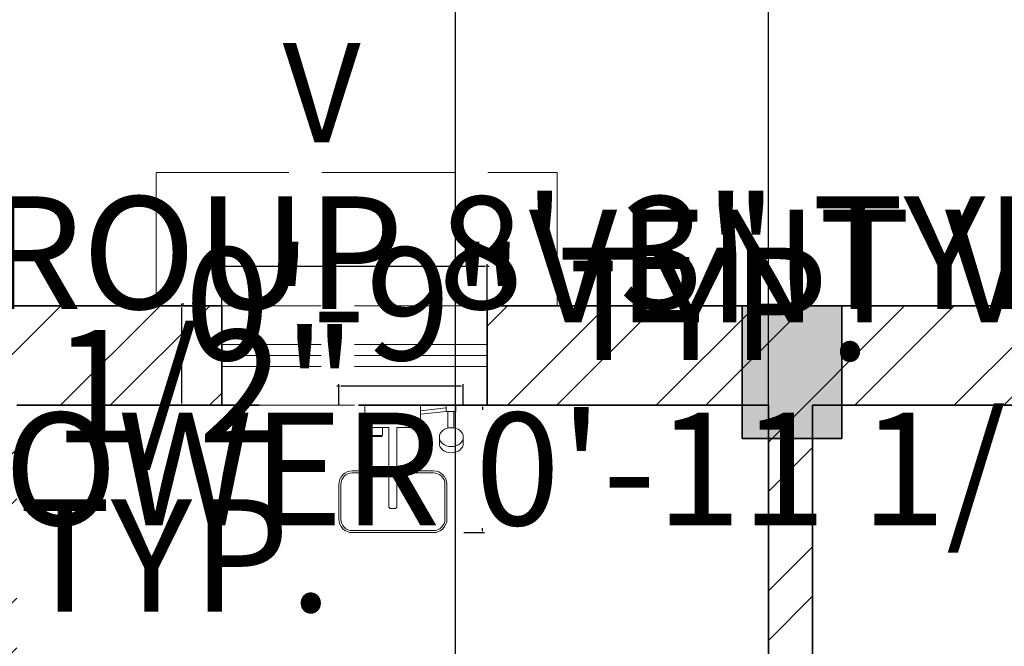
# Model space of a CAD drawing. Units: inches. Extents: x 2379 to 3013, y 1431 to 2110.
# Tile 7 of 10: x 2696 to 2785, y 1991 to 2047. Entities that reach past the tile are written whole.
import ezdxf

# ---------------------------------------------------------------- set-up
doc = ezdxf.new("R2010")
doc.units = ezdxf.units.IN
doc.linetypes.add('ACAD_ISO02W100', pattern=[15, 12, -3])
for name, color, linetype, lineweight in [('A-ANNO-DIMS', 2, 'Continuous', 18), ('A-ANNO-TEXT', 7, 'Continuous', 18), ('A-COLS', 7, 'Continuous', 35), ('A-COLS-PATT', 252, 'Continuous', 13), ('A-FLOR-FIXT', 9, 'Continuous', 18), ('A-GLAZ-VENT', 6, 'ACAD_ISO02W100', 13), ('A-ROOF-OVHD', 11, 'ACAD_ISO02W100', 13), ('A-WALL-PATT', 8, 'Continuous', 13), ('WALL', 7, 'Continuous', 35)]:
    doc.layers.add(name, color=color, linetype=linetype, lineweight=lineweight)
doc.styles.get("Standard").update_dxf_attribs({"font": 'arial.ttf'})
doc.dimstyles.get("Standard").update_dxf_attribs({"dimtxt": 10.18, "dimasz": 0.18, "dimexe": 0.18, "dimexo": 0.0625, "dimgap": 0.09, "dimtad": 0, "dimtih": 1, "dimtoh": 1, "dimdec": 0, "dimzin": 0, "dimdsep": 46, "dimlunit": 3, "dimtxsty": 'Standard', "dimcen": 0.09, "dimadec": 0, "dimazin": 0, "dimtfac": 1, "dimtdec": 0, "dimtofl": 0, "dimtmove": 0, "dimatfit": 3, "dimfxl": 1, "dimtolj": 1, "dimtzin": 0, "dimarcsym": 0})

# ---------------------------------------------------------------- blocks, each defined once
blk = doc.blocks.new('column')
for p, q in [((2588.21307907444, 2021.786762638958), (2597.21307907444, 2021.786762638958)), ((2588.21307907444, 2009.786762638958), (2588.21307907444, 2021.786762638958)), ((2597.21307907444, 2021.786762638958), (2597.21307907444, 2009.786762638958)), ((2597.21307907444, 2009.786762638958), (2588.21307907444, 2009.786762638958))]:
    blk.add_line(p, q)
blk = doc.blocks.new('A$C7A0926BE')
for p, q in [((-6.551239185704615, 4.547e-13), (-5.566804685018722, 4.547e-13)), ((-6.551239185704615, -0.6519594773226345), (-6.551239185704615, 4.547e-13)), ((-5.566804685018722, 4.547e-13), (-5.566804685018722, -0.6519594773226345)), ((-2.885464417704497, 4.547e-13), (-2.885464417704497, -2.294617439688408)), ((2.885464417697221, 4.547e-13), (-2.885464417704497, 4.547e-13)), ((2.885464417697221, -2.294617439688408), (2.885464417697221, 4.547e-13)), ((-5.566804685018722, -0.6519594773226345), (-6.551239185704615, -0.6519594773226345)), ((-6.337339280165905, -0.6519594773226345), (-5.736871956549292, -0.6519594773226345)), ((-6.337339280165905, -2.331605676014532), (-6.337339280165905, -0.6519594773226345)), ((-5.736871956549292, -0.6519594773226345), (-5.736871956549292, -2.331605676014532)), ((-5.566804685018722, -0.2752176342105486), (-2.885464417704497, -0.5594689734662098)), ((-5.566804685018722, -0.6519594773226345), (-2.885464417704497, -0.9362108165782956)), ((-5.736871956549292, -2.331605676014532), (-6.337339280165905, -2.331605676014532)), ((-2.885464417704497, -2.294617439688408), (-0.4493639847714804, -2.294617439688408)), ((0.3906360152323032, -2.294617439688408), (2.885464417697221, -2.294617439688408)), ((1.037687122458008, -2.294617439688408), (1.037687122458008, -3.123877501528568)), ((2.370543453427671, -2.294617439688408), (1.037687122458008, -2.294617439688408)), ((2.370543453427671, -3.123877501528568), (2.370543453427671, -2.294617439688408)), ((-7.324834426704909, -3.292217109228203), (-7.324834426704909, -3.941342171486666)), ((-4.843765035140676, -3.941342171486666), (-4.849446849475498, -3.292217109228203)), ((1.037687122458008, -3.123877501528568), (2.370543453427671, -3.123877501528568)), ((1.127016126156376, -3.123877501528568), (1.127016126156376, -3.234129205485259)), ((2.303627794695784, -3.123877501528568), (1.127016126156376, -3.123877501528568)), ((1.127016126156376, -3.234129205485259), (2.303627794695784, -3.234129205485259)), ((2.303627794695784, -3.234129205485259), (2.303627794695784, -3.123877501528568))]:
    blk.add_line(p, q)
at = {"ltscale": 100}
for p, q in [((-0.4493639847642045, -10.48461743968892), (-0.4493639847714804, -2.294617439688408)), ((0.3906360152323032, -10.48461743968892), (0.3906360152323032, -2.294617439688408)), ((0.1806360152259003, -10.6946174396885), (-0.2393639847723534, -10.6946174396885))]:
    blk.add_line(p, q, dxfattribs=at)
for points in [[(-0.4493639847642045, -6.794023881873727), (-4.22936398476304, -6.794023881873727, 0.4142135623730951), (-5.629363984764494, -8.194023881873362), (-5.629363984764494, -11.79521099750036, 0.4142135623730951), (-4.22936398476304, -13.19521099750091), (4.170636015231138, -13.19521099750091, 0.4142135623730951), (5.570636015232594, -11.79521099750036), (5.570636015232594, -8.194023881873362, 0.4142135623730951), (4.170636015231138, -6.794023881873727), (0.3906360152323032, -6.794023881873727)], [(-0.4493639847642045, -7.004023881873306), (-4.22936398476304, -7.004023881873306, 0.4142135623733461), (-5.419363984772644, -8.194023881873362), (-5.419363984772644, -11.79521099750036, 0.4142135623733461), (-4.22936398476304, -12.98521099750132), (4.170636015231138, -12.98521099750132, 0.4142135623733461), (5.360636015233466, -11.79521099750036), (5.360636015233466, -8.194023881873362, 0.4142135623733461), (4.170636015231138, -7.004023881873306), (0.3906360152323032, -7.004023881873306)]]:
    blk.add_lwpolyline(points, format="xyb", dxfattribs=at)
for centre, start, end in [((-0.2393639847723534, -10.48461743968892), 180, 270), ((0.1806360152259003, -10.48461743968892), 270, 0)]:
    blk.add_arc(centre, 0.2099999999999999, start, end, dxfattribs=at)
at = {"extrusion": (0, 0, -1)}
blk.add_ellipse((-6.084299730922793, -3.292217109228203), major_axis=(-1.240534695781024, -2.0763e-12), ratio=0.7908490116437874, dxfattribs=at)
blk.add_ellipse((-6.084299730922793, -3.941342171486666), major_axis=(-1.240534695781024, -1.4783e-12), ratio=0.7908490116437878, start_param=3.141592653591299, end_param=6.283185307181092, dxfattribs=at)
blk = doc.blocks.new('*D14')
at = {"layer": 'A-ANNO-DIMS', "color": 0, "lineweight": -2, "transparency": 16777216}
for p, q in [((2469.628133617025, 2021.670980178146), (2469.628133617025, 2076.343811217002)), ((2937.628133542687, 2021.670980178146), (2937.628133542687, 2076.343811217002)), ((2469.808133617025, 2076.163811217002), (2694.903188150115, 2076.163811217002)), ((2937.448133542687, 2076.163811217002), (2712.353079009597, 2076.163811217002))]:
    blk.add_line(p, q, dxfattribs=at)
at = {"layer": 'A-ANNO-DIMS', "color": 0, "transparency": 16777216}
for points in [[(2469.808133617025, 2076.193811217002), (2469.808133617025, 2076.133811217002), (2469.628133617025, 2076.163811217002)], [(2937.448133542687, 2076.193811217002), (2937.448133542687, 2076.133811217002), (2937.628133542687, 2076.163811217002)]]:
    blk.add_solid(points, dxfattribs=at)
at = {"layer": 'Defpoints', "color": 0, "transparency": 16777216}
for p in [(2937.628133542687, 2076.163811217002), (2469.628133617025, 2021.608480178145), (2937.628133542687, 2021.608480178146)]:
    blk.add_point(p, dxfattribs=at)
at = {"layer": 'A-ANNO-DIMS', "color": 0, "transparency": 16777216, "insert": (2703.628133579856, 2076.163811217002), "char_height": 10.18, "attachment_point": 5}
blk.add_mtext("\\A1;39'", dxfattribs=at)
blk = doc.blocks.new('VENT-24IN')
for p, q in [((23.99961244475026, 5.50048129934089), (-0.0003875552497448, 5.50048129934089)), ((23.99961244475026, 4.50048129934089), (-0.0003875552497448, 4.50048129934089)), ((23.99961244475026, 3.50048129934089), (-0.0003875552497448, 3.50048129934089))]:
    blk.add_line(p, q)
blk.add_lwpolyline([(-0.0003875552497448, 9.00048129910806), (-0.0003875552497448, 0.0004812991080598), (23.99961244475026, 0.0004812993408905), (23.99961244475026, 9.00048129934089)], close=True)
blk = doc.blocks.new('*D26')
at = {"layer": 'A-ANNO-DIMS', "color": 0, "lineweight": -2, "transparency": 16777216}
for p, q in [((2688.622898699378, 1958.67097978589), (2688.622898699378, 1963.759108581785)), ((2688.802898699378, 1963.579108581785), (2721.580424005343, 1963.579108581785)), ((2721.760424005343, 1958.67097978589), (2721.760424005343, 1963.759108581785)), ((2721.760424005343, 1963.579108581785), (2721.940424005343, 1963.579108581785))]:
    blk.add_line(p, q, dxfattribs=at)
at = {"layer": 'A-ANNO-DIMS', "color": 0, "transparency": 16777216}
for points in [[(2688.802898699378, 1963.609108581785), (2688.802898699378, 1963.549108581785), (2688.622898699378, 1963.579108581785)], [(2721.580424005343, 1963.609108581785), (2721.580424005343, 1963.549108581785), (2721.760424005343, 1963.579108581785)]]:
    blk.add_solid(points, dxfattribs=at)
at = {"layer": 'Defpoints', "color": 0, "transparency": 16777216}
for p in [(2721.760424005343, 1963.579108581785), (2688.622898699378, 1958.60847978589), (2721.760424005343, 1958.60847978589)]:
    blk.add_point(p, dxfattribs=at)
at = {"layer": 'A-ANNO-DIMS', "color": 0, "transparency": 16777216, "insert": (2787.176174346408, 1963.579108581785), "char_height": 10.18, "attachment_point": 5}
blk.add_mtext('\\A1;DOOR D1 2\'-9" TYP.', dxfattribs=at)
blk = doc.blocks.new('*D28')
at = {"layer": 'A-ANNO-DIMS', "color": 0, "lineweight": -2, "transparency": 16777216}
for p, q in [((2714.172792821913, 2021.670981299344), (2714.172792821913, 2025.388481299344)), ((2714.352792821913, 2025.208481299344), (2737.992792821913, 2025.208481299344)), ((2738.172792821913, 2021.670981299344), (2738.172792821913, 2025.388481299344)), ((2738.172792821913, 2025.208481299344), (2738.352792821912, 2025.208481299344))]:
    blk.add_line(p, q, dxfattribs=at)
at = {"layer": 'A-ANNO-DIMS', "color": 0, "transparency": 16777216}
for points in [[(2714.352792821913, 2025.238481299344), (2714.352792821913, 2025.178481299344), (2714.172792821913, 2025.208481299344)], [(2737.992792821913, 2025.238481299344), (2737.992792821913, 2025.178481299344), (2738.172792821913, 2025.208481299344)]]:
    blk.add_solid(points, dxfattribs=at)
at = {"layer": 'Defpoints', "color": 0, "transparency": 16777216}
for p in [(2738.172792821913, 2025.208481299344), (2714.172792821913, 2021.608481299344), (2738.172792821913, 2021.608481299344)]:
    blk.add_point(p, dxfattribs=at)
at = {"layer": 'A-ANNO-DIMS', "color": 0, "transparency": 16777216, "insert": (2797.390964718229, 2025.208481299344), "char_height": 10.18, "attachment_point": 5}
blk.add_mtext('\\A1;VENT V 2\'-0" TYP.', dxfattribs=at)
blk = doc.blocks.new('*D29')
at = {"layer": 'A-ANNO-DIMS', "color": 0, "lineweight": -2, "transparency": 16777216}
for p, q in [((2714.110292821914, 2021.608481299345), (2710.392792821915, 2021.608481299345)), ((2710.572792821915, 2021.608481299345), (2710.572792821915, 2021.788481299345)), ((2710.572792821915, 2021.788481299345), (2710.752792821915, 2021.788481299345)), ((2710.572792821915, 2012.788481299112), (2710.572792821915, 2021.428481299345)), ((2714.110292821914, 2012.608481299112), (2710.392792821915, 2012.608481299112))]:
    blk.add_line(p, q, dxfattribs=at)
at = {"layer": 'A-ANNO-DIMS', "color": 0, "transparency": 16777216}
for points in [[(2710.542792821915, 2021.428481299345), (2710.602792821915, 2021.428481299345), (2710.572792821915, 2021.608481299345)], [(2710.542792821915, 2012.788481299112), (2710.602792821915, 2012.788481299112), (2710.572792821915, 2012.608481299112)]]:
    blk.add_solid(points, dxfattribs=at)
at = {"layer": 'Defpoints', "color": 0, "transparency": 16777216}
for p in [(2710.572792821915, 2021.608481299345), (2714.172792821913, 2021.608481299345), (2714.172792821913, 2012.608481299112)]:
    blk.add_point(p, dxfattribs=at)
at = {"layer": 'A-ANNO-DIMS', "color": 0, "transparency": 16777216, "insert": (2741.868877405817, 2021.788481299344), "char_height": 10.18, "attachment_point": 5}
blk.add_mtext('\\A1;0\'-9" TYP.', dxfattribs=at)
blk = doc.blocks.new('*D30')
at = {"layer": 'A-ANNO-DIMS', "color": 0, "lineweight": -2, "transparency": 16777216}
for p, q in [((2800.258423213022, 2011.627222646179), (2800.258423213022, 2026.594722646179)), ((2899.258423213023, 2011.627222646179), (2899.258423213023, 2026.594722646179)), ((2800.258423213022, 2026.414722646178), (2800.078423213022, 2026.414722646178)), ((2899.078423213023, 2026.414722646178), (2800.438423213022, 2026.414722646178))]:
    blk.add_line(p, q, dxfattribs=at)
at = {"layer": 'A-ANNO-DIMS', "color": 0, "transparency": 16777216}
for points in [[(2800.438423213022, 2026.444722646179), (2800.438423213022, 2026.384722646179), (2800.258423213022, 2026.414722646178)], [(2899.078423213023, 2026.444722646179), (2899.078423213023, 2026.384722646179), (2899.258423213023, 2026.414722646178)]]:
    blk.add_solid(points, dxfattribs=at)
at = {"layer": 'Defpoints', "color": 0, "transparency": 16777216}
for p in [(2800.258423213022, 2026.414722646178), (2800.258423213022, 2011.564722646179), (2899.258423213023, 2011.564722646179)]:
    blk.add_point(p, dxfattribs=at)
at = {"layer": 'A-ANNO-DIMS', "color": 0, "transparency": 16777216, "insert": (2724.541151725982, 2026.414722646178), "char_height": 10.18, "attachment_point": 5}
blk.add_mtext('\\A1;BED GROUP 8\'-3" TYP.', dxfattribs=at)
blk = doc.blocks.new('*D40')
at = {"layer": 'A-ANNO-DIMS', "color": 0, "lineweight": -2, "transparency": 16777216}
for p, q in [((2676.995321732777, 2012.608480178204), (2681.188134232791, 2012.608480178204)), ((2681.008134232791, 2012.428480178203), (2681.008134232791, 2004.381178848007)), ((2681.008134232791, 1985.619730178112), (2681.008134232791, 1993.667031508307)), ((2676.995321732777, 1985.439730178112), (2681.188134232791, 1985.439730178112))]:
    blk.add_line(p, q, dxfattribs=at)
at = {"layer": 'A-ANNO-DIMS', "color": 0, "transparency": 16777216}
for points in [[(2680.978134232791, 2012.428480178203), (2681.038134232792, 2012.428480178203), (2681.008134232791, 2012.608480178204)], [(2680.978134232791, 1985.619730178112), (2681.038134232792, 1985.619730178112), (2681.008134232791, 1985.439730178112)]]:
    blk.add_solid(points, dxfattribs=at)
at = {"layer": 'Defpoints', "color": 0, "transparency": 16777216}
for p in [(2676.932821732777, 2012.608480178204), (2681.008134232791, 2012.608480178204), (2676.932821732777, 1985.439730178112)]:
    blk.add_point(p, dxfattribs=at)
at = {"layer": 'A-ANNO-DIMS', "color": 0, "transparency": 16777216, "insert": (2681.008134232791, 1999.024105178156), "char_height": 10.18, "attachment_point": 5}
blk.add_mtext('\\A1;WC 2\'-3" TYP.', dxfattribs=at)
blk = doc.blocks.new('*D46')
at = {"layer": 'A-ANNO-DIMS', "color": 0, "lineweight": -2, "transparency": 16777216}
for p, q in [((2736.087387447885, 2012.608480178147), (2737.933387607347, 2012.608480178147)), ((2737.753387607348, 2012.428480178146), (2737.753387607348, 2012.203886649792)), ((2737.753387607348, 2001.265145781737), (2737.753387607348, 2001.489739310092)), ((2736.087387447885, 2001.085145781737), (2737.933387607347, 2001.085145781737))]:
    blk.add_line(p, q, dxfattribs=at)
at = {"layer": 'A-ANNO-DIMS', "color": 0, "transparency": 16777216}
for points in [[(2737.723387607348, 2012.428480178146), (2737.783387607348, 2012.428480178146), (2737.753387607348, 2012.608480178147)], [(2737.723387607348, 2001.265145781737), (2737.783387607348, 2001.265145781737), (2737.753387607348, 2001.085145781737)]]:
    blk.add_solid(points, dxfattribs=at)
at = {"layer": 'Defpoints', "color": 0, "transparency": 16777216}
for p in [(2736.024887447885, 2012.608480178147), (2737.753387607348, 2012.608480178147), (2736.024887447885, 2001.085145781737)]:
    blk.add_point(p, dxfattribs=at)
at = {"layer": 'A-ANNO-DIMS', "color": 0, "transparency": 16777216, "insert": (2737.753387607348, 2006.84681297994), "char_height": 10.18, "attachment_point": 5}
blk.add_mtext('\\A1;SHOWER 0\'-11 1/2"', dxfattribs=at)
blk = doc.blocks.new('*D47')
at = {"layer": 'A-ANNO-DIMS', "color": 0, "lineweight": -2, "transparency": 16777216}
for p, q in [((2724.763315493515, 2014.336980337607), (2724.583315493515, 2014.336980337607)), ((2724.763315493515, 2012.670980178146), (2724.763315493515, 2014.516980337607)), ((2735.844887447885, 2014.336980337607), (2724.943315493514, 2014.336980337607)), ((2736.024887447884, 2012.670980178146), (2736.024887447884, 2014.516980337607))]:
    blk.add_line(p, q, dxfattribs=at)
at = {"layer": 'A-ANNO-DIMS', "color": 0, "transparency": 16777216}
for points in [[(2724.943315493514, 2014.366980337607), (2724.943315493514, 2014.306980337607), (2724.763315493515, 2014.336980337607)], [(2735.844887447885, 2014.366980337607), (2735.844887447885, 2014.306980337607), (2736.024887447884, 2014.336980337607)]]:
    blk.add_solid(points, dxfattribs=at)
at = {"layer": 'Defpoints', "color": 0, "transparency": 16777216}
for p in [(2724.763315493515, 2014.336980337607), (2724.763315493515, 2012.608480178146), (2736.024887447884, 2012.608480178146)]:
    blk.add_point(p, dxfattribs=at)
at = {"layer": 'A-ANNO-DIMS', "color": 0, "transparency": 16777216, "insert": (2695.147694756816, 2014.336980337607), "char_height": 10.18, "attachment_point": 5}
blk.add_mtext('\\A1;0\'-11 1/2"', dxfattribs=at)
blk = doc.blocks.new('*D65')
at = {"layer": 'A-ANNO-DIMS', "color": 0, "lineweight": -2, "transparency": 16777216}
for p, q in [((2735.322583, 1920.855034), (2735.322583, 2094.642393)), ((2735.502583, 2094.462393), (2763.448134000001, 2094.462393)), ((2763.628134, 1924.67098), (2763.628134, 2094.642393)), ((2763.628134, 2094.462393), (2763.808134, 2094.462393))]:
    blk.add_line(p, q, dxfattribs=at)
at = {"layer": 'A-ANNO-DIMS', "color": 0, "transparency": 16777216}
for points in [[(2735.502583, 2094.492393), (2735.502583, 2094.432392999999), (2735.322583, 2094.462393)], [(2763.448134000001, 2094.492393), (2763.448134000001, 2094.432392999999), (2763.628134, 2094.462393)]]:
    blk.add_solid(points, dxfattribs=at)
at = {"layer": 'Defpoints', "color": 0, "transparency": 16777216}
for p in [(2763.628134, 2094.462393), (2763.628134, 1924.60848), (2735.322583, 1920.792534)]:
    blk.add_point(p, dxfattribs=at)
at = {"layer": 'A-ANNO-DIMS', "color": 0, "transparency": 16777216, "insert": (2789.375910261937, 2094.462393), "char_height": 10.18, "attachment_point": 5}
blk.add_mtext('\\A1;2\'-4 1/2"', dxfattribs=at)

msp = doc.modelspace()

# ---------------------------------------------------------------- hatches: boundary and pattern name
at = {"layer": 'A-COLS-PATT'}
h = msp.add_hatch(color=256, dxfattribs=at)
h.dxf.hatch_style = 1
h.paths.add_polyline_path([(2937.622722034017, 1660.608479805985), (2925.622722034017, 1660.608479805985), (2925.622722034017, 1651.608480178145), (2937.622722034017, 1651.608480178145)])
h.paths.add_polyline_path([(2481.628132350232, 1809.608480178145), (2478.628133617025, 1809.608480178145), (2478.628133617025, 1811.017018303813), (2469.628133617025, 1811.017018303813), (2469.628133617025, 1802.017018303813), (2478.628133617025, 1802.017018303813), (2478.628133617025, 1805.608480178145), (2481.628132350232, 1805.608480178145)])
h.paths.add_polyline_path([(2481.628132350232, 1811.017018303813), (2478.628133617025, 1811.017018303813), (2478.628133617025, 1809.608480178145), (2481.628132350232, 1809.608480178145)], flags=17)
h.paths.add_polyline_path([(2481.628132350232, 1805.608480178145), (2478.628133617025, 1805.608480178145), (2478.628133617025, 1802.017018303813), (2481.628132350232, 1802.017018303813)], flags=17)
h.paths.add_polyline_path([(2481.628132350232, 1660.608479805985), (2469.628133617025, 1660.608479805985), (2469.628133617025, 1651.608480178145), (2481.628132350232, 1651.608480178145)])
h.paths.add_polyline_path([(2692.072955574556, 1660.608480178145), (2688.628133617025, 1660.608480178145), (2688.628133617025, 1663.608479805985), (2684.628133617025, 1663.608479805985), (2684.628133617025, 1660.608480178145), (2683.072955574556, 1660.608480178145), (2683.072955574556, 1651.608480178145), (2692.072955574556, 1651.608480178145)])
h.paths.add_polyline_path([(2692.072955574556, 1663.608479805985), (2688.628133617025, 1663.608479805985), (2688.628133617025, 1660.608480178145), (2692.072955574556, 1660.608480178145)], flags=17)
h.paths.add_polyline_path([(2684.628133617025, 1663.608479805985), (2683.072955574556, 1663.608479805985), (2683.072955574556, 1660.608480178145), (2684.628133617025, 1660.608480178145)], flags=17)
h.paths.add_polyline_path([(2770.631540519471, 1660.608480178145), (2767.628133617025, 1660.608480178145), (2767.628133617025, 1663.608479805985), (2763.628133617025, 1663.608479805985), (2763.628133617025, 1660.608480178145), (2761.631540519471, 1660.608480178145), (2761.631540519471, 1651.608480178145), (2763.628133617025, 1651.608480178145), (2767.628133617026, 1651.608479965586), (2767.628133617026, 1651.608480178145), (2770.631540519471, 1651.608480178145)])
h.paths.add_polyline_path([(2770.631540519471, 1663.608479805985), (2767.628133617025, 1663.608479805985), (2767.628133617025, 1660.608480178145), (2770.631540519471, 1660.608480178145)], flags=17)
h.paths.add_polyline_path([(2763.628133617025, 1663.608479805985), (2761.631540519471, 1663.608479805985), (2761.631540519471, 1660.608480178145), (2763.628133617025, 1660.608480178145)], flags=17)
h.paths.add_polyline_path([(2937.628133617025, 1813.620125754823), (2928.628133617025, 1813.620125754823), (2928.628133617025, 1810.608480178145), (2925.628133617025, 1810.608480178145), (2925.628133617025, 1806.608480178145), (2928.628133617025, 1806.608480178145), (2928.628133617025, 1804.620125754824), (2937.628133617025, 1804.620125754824)], flags=17)
h.paths.add_polyline_path([(2937.628133617025, 1813.620125754823), (2928.628133617025, 1813.620125754823), (2928.628133617025, 1810.608480178145), (2925.628133617025, 1810.608480178145), (2925.628133617025, 1804.620125754824), (2937.628133617025, 1804.620125754824)], flags=17)
h.paths.add_polyline_path([(2928.628133617025, 1813.620125754823), (2925.628133617025, 1813.620125754823), (2925.628133617025, 1810.608480178145), (2928.628133617025, 1810.608480178145)], flags=0)
h.paths.add_polyline_path([(2937.628133617025, 1863.796245476747), (2928.628133617026, 1863.796245476747), (2928.628133617026, 1862.608480178145), (2925.628133617025, 1862.608480178145), (2925.628133617025, 1858.608480178145), (2928.628133617026, 1858.608480178145), (2928.628133617026, 1854.796245476746), (2937.628133617025, 1854.796245476746)])
h.paths.add_polyline_path([(2928.628133617026, 1863.796245476747), (2925.628133617025, 1863.796245476747), (2925.628133617025, 1862.608480178145), (2928.628133617026, 1862.608480178145)], flags=17)
h.paths.add_polyline_path([(2928.628133617026, 1858.608480178145), (2925.628133617025, 1858.608480178145), (2925.628133617025, 1854.796245476746), (2928.628133617026, 1854.796245476746)], flags=17)
h.paths.add_polyline_path([(2937.628133542687, 2021.608480178145), (2928.628133542687, 2021.608480178145), (2928.628133542687, 2012.608480178145), (2928.628133617026, 2012.608480178145), (2928.628133617026, 2009.608480178145), (2937.628133542687, 2009.608480178145)])
h.paths.add_polyline_path([(2770.26658329333, 2021.608480178145), (2761.26658329333, 2021.608480178145), (2761.26658329333, 2012.608480178145), (2763.628133617026, 2012.608480178145), (2763.628133617026, 2009.608480178145), (2767.628133617026, 2009.608480178145), (2767.628133617026, 2012.608480178145), (2770.26658329333, 2012.608480178145)])
h.paths.add_polyline_path([(2763.628133617026, 2012.608480178145), (2761.26658329333, 2012.608480178145), (2761.26658329333, 2009.608480178145), (2763.628133617026, 2009.608480178145)], flags=17)
h.paths.add_polyline_path([(2770.26658329333, 2012.608480178145), (2767.628133617026, 2012.608480178145), (2767.628133617026, 2009.608480178145), (2770.26658329333, 2009.608480178145)], flags=17)
h.paths.add_polyline_path([(2597.21307907444, 2021.608480178145), (2588.21307907444, 2021.608480178145), (2588.21307907444, 2012.608480178145), (2590.628133617026, 2012.608480178145), (2590.628133617026, 2009.608480178145), (2594.628133617025, 2009.608480178145), (2594.628133617025, 2012.608480178145), (2597.21307907444, 2012.608480178145)])
h.paths.add_polyline_path([(2590.628133617026, 2012.608480178145), (2588.21307907444, 2012.608480178145), (2588.21307907444, 2009.608480178145), (2590.628133617026, 2009.608480178145)], flags=17)
h.paths.add_polyline_path([(2597.21307907444, 2012.608480178145), (2594.628133617025, 2012.608480178145), (2594.628133617025, 2009.608480178145), (2597.21307907444, 2009.608480178145)], flags=17)
at = {"layer": 'A-WALL-PATT'}
h = msp.add_hatch(dxfattribs=at)
h.set_pattern_fill('ANSI32', color=256)
h.set_pattern_definition([(45, (0, 0), (-6.735192090801865, 6.735192090801866), []), (45, (4.49013, 0), (-6.735192090801865, 6.735192090801866), [])])
h.paths.add_polyline_path([(2925.628133617025, 1862.608480178145), (2815.628133617027, 1862.608480178145), (2815.628133617026, 1858.608480178145), (2827.628133617026, 1858.608480178145), (2827.62813361702, 1810.608480178145), (2815.628133617021, 1810.608480178145), (2815.62813361702, 1806.608480178145), (2850.776028957045, 1806.608480178145), (2850.776028957045, 1810.608480178145), (2831.628133617021, 1810.608480178145), (2831.628133617026, 1858.608480178145), (2925.628133617025, 1858.608480178145)])
h.paths.add_polyline_path([(2925.628133617025, 1810.608480178145), (2880.776028957045, 1810.608480178145), (2880.776028957046, 1806.608480178145), (2925.628133617025, 1806.608480178145)], flags=17)
h.paths.add_polyline_path([(2633.752023401108, 1660.608480178145), (2594.628133617026, 1660.608480178145), (2481.628132350232, 1660.608480178145), (2481.628132350232, 1651.608480178145), (2588.628133617025, 1651.608480178145), (2588.628133617025, 1570.608480178146), (2624.284264477168, 1570.608480178146), (2624.284264477168, 1574.608480178146), (2592.628133617025, 1574.608480178146), (2592.628133617025, 1651.608480178145), (2633.752023401108, 1651.608480178145)])
h.paths.add_polyline_path([(2594.628133617025, 1809.608480178145), (2481.628132350232, 1809.608480178145), (2481.628132350232, 1805.608480178145), (2594.628133617025, 1805.608480178145)])
h.paths.add_polyline_path([(2594.628133617025, 2012.608480178145), (2597.21307907444, 2012.608480178145), (2597.21307907444, 2021.608480178145), (2588.21307907444, 2021.608480178145), (2588.21307907444, 2012.608480178145), (2590.628133617026, 2012.608480178145), (2590.628133617025, 1845.608480178145), (2594.628133617025, 1845.608480178145)])
h.paths.add_polyline_path([(2767.628133617026, 2012.608480178145), (2770.26658329333, 2012.608480178145), (2770.26658329333, 2021.608480178145), (2761.26658329333, 2021.608480178145), (2761.26658329333, 2012.608480178145), (2763.628133617026, 2012.608480178145), (2763.628133617026, 1928.608480178145), (2691.628133617026, 1928.608480178146), (2643.628133617026, 1928.608480178146), (2643.628133617026, 1924.608480178146), (2691.628133617026, 1924.608480178145), (2763.628133617026, 1924.608480178145), (2763.628133617026, 1858.608480178145), (2779.628133617026, 1858.608480178145), (2779.628133617026, 1862.608480178145), (2767.628133617026, 1862.608480178145)])
h.paths.add_polyline_path([(2613.628133617026, 2012.608480178146), (2613.628133617026, 2021.608480178145), (2597.21307907444, 2021.608480178145), (2597.21307907444, 2012.608480178145)])
h.paths.add_polyline_path([(2508.325157742558, 2012.608480178146), (2508.325157742557, 2021.608480178145), (2478.628133617025, 2021.608480178145), (2478.628133617025, 2012.608480178145)])
h.paths.add_polyline_path([(2556.325157742558, 2021.608480178145), (2556.325157742558, 2012.608480178145), (2588.21307907444, 2012.608480178145), (2588.21307907444, 2021.608480178145)])
h.paths.add_polyline_path([(2659.149603475649, 2012.608480178146), (2659.149603475649, 2021.608480178145), (2643.628133617026, 2021.608480178145), (2643.628133617025, 1958.608480178146), (2661.628133617025, 1958.608480178146), (2661.628133617026, 1962.608480178146), (2647.628133617026, 1962.608480178146), (2647.628133617026, 2012.608480178145)])
h.paths.add_polyline_path([(2714.172783852811, 2012.608480178145), (2714.172783852811, 2021.608480178145), (2683.149603475648, 2021.608480178145), (2683.149603475648, 2012.608480178145), (2691.628133617026, 2012.608480178145), (2691.628133617026, 1958.608480178146), (2695.628133617026, 1958.608480178146), (2695.628133617026, 2012.608480178145)])
h.paths.add_polyline_path([(2738.172783852812, 2021.608480178145), (2738.172783852811, 2012.608480178145), (2761.26658329333, 2012.608480178145), (2761.26658329333, 2021.608480178145)])
h.paths.add_polyline_path([(2820.757909975796, 2012.608480178145), (2820.757909975796, 2021.608480178145), (2770.26658329333, 2021.608480178145), (2770.26658329333, 2012.608480178145)])
h.paths.add_polyline_path([(2868.757909975796, 2021.608480178145), (2868.757909975795, 2012.608480178145), (2928.628133542687, 2012.608480178145), (2928.628133542687, 2021.608480178145)])
h.paths.add_polyline_path([(2928.628133617026, 1962.897453102627), (2937.628133617025, 1962.897453102627), (2937.628133617025, 2009.608480178145), (2928.628133617026, 2009.608480178145)])
h.paths.add_polyline_path([(2937.628133617025, 1914.897453102627), (2928.628133617026, 1914.897453102627), (2928.628133617026, 1863.796245476747), (2937.628133617025, 1863.796245476747)])
h.paths.add_polyline_path([(2928.628133617025, 1846.587382132453), (2937.628133617025, 1846.587382132453), (2937.628133617025, 1854.796245476746), (2928.628133617026, 1854.796245476746)])
h.paths.add_polyline_path([(2937.628133617025, 1822.587382132453), (2928.628133617025, 1822.587382132453), (2928.628133617025, 1813.620125754823), (2937.628133617025, 1813.620125754823)])
h.paths.add_polyline_path([(2928.628133617025, 1778.475127785104), (2937.628133617026, 1778.475127785104), (2937.628133617025, 1813.620125754823), (2928.628133617025, 1813.620125754823), (2928.628133617025, 1810.608480178145), (2925.628133617025, 1810.608480178145), (2925.628133617025, 1806.608480178145), (2928.628133617025, 1806.608480178145)])
h.paths.add_polyline_path([(2816.219214803751, 1651.608480178145), (2816.219214803751, 1660.608480178145), (2767.628133617025, 1660.608480178145), (2767.628133617025, 1806.608480178145), (2779.62813361702, 1806.608480178145), (2779.62813361702, 1810.608480178145), (2763.628133617026, 1810.608480178145), (2763.628133617025, 1660.608480178145), (2688.628133617025, 1660.608480178145), (2688.628133617026, 1810.608480178144), (2684.628133617026, 1810.608480178145), (2684.628133617025, 1660.608480178145), (2669.752023401108, 1660.608480178145), (2669.752023401108, 1651.608480178145), (2763.628133617025, 1651.608480178145), (2763.628133617025, 1574.608480178145), (2672.284264477169, 1574.608480178145), (2672.284264477168, 1570.608480178145), (2767.628133617026, 1570.608480178145), (2767.628133617026, 1651.608480178145)])
h.paths.add_polyline_path([(2864.219214803751, 1660.608480178145), (2864.219214803751, 1651.608480178145), (2937.628133617025, 1651.608480178145), (2937.628133617026, 1730.475127785104), (2928.628133617025, 1730.475127785104), (2928.628133617025, 1660.608480178145)])
h.paths.add_polyline_path([(2469.628133617026, 1975.187574086886), (2478.628133617025, 1975.187574086886), (2478.628133617025, 2009.608480178146), (2469.628133617025, 2009.608480178146)])
h.paths.add_polyline_path([(2478.628133617025, 1927.187574086886), (2469.628133617026, 1927.187574086886), (2469.628133617025, 1811.017018303813), (2478.628133617025, 1811.017018303813)])
h.paths.add_polyline_path([(2469.628133617025, 1758.038369990633), (2478.628133617025, 1758.038369990633), (2478.628133617025, 1802.017018303813), (2469.628133617025, 1802.017018303813)])
h.paths.add_polyline_path([(2478.628133617025, 1710.038369990633), (2469.628133617025, 1710.038369990633), (2469.628133617025, 1660.608479805985), (2478.628133617025, 1660.608479805985)])

# ---------------------------------------------------------------- linework, layer by layer
at = {"layer": 'A-ROOF-OVHD'}
for p, q in [((2708.241503463928, 2021.608480178145), (2708.241503463928, 2033.666337873881)), ((2708.241503463928, 2033.666337873881), (2744.51533817465, 2033.666337873881)), ((2744.51533817465, 2033.666337873881), (2744.515338174651, 2021.608480178145))]:
    msp.add_line(p, q, dxfattribs=at)
at = {"layer": 'WALL'}
for p, q in [((2683.149603475648, 2021.608480178145), (2714.172783852811, 2021.608480178145)), ((2714.172783852811, 2012.608480178145), (2714.172783852811, 2021.608480178145)), ((2738.172783852811, 2012.608480178145), (2738.172783852811, 2021.608480178145)), ((2738.172783852811, 2021.608480178145), (2820.757909975796, 2021.608480178145)), ((2695.628133617026, 2012.608480178145), (2717.55858762154, 2012.608480178145)), ((2726.538841803143, 2012.608480178145), (2763.628133617026, 2012.608480178145)), ((2744.51533817465, 2012.624462368048), (2744.51533817465, 2012.608480178145)), ((2763.628133617026, 2012.608480178146), (2763.628133617026, 1928.608480178145)), ((2767.628133617026, 2012.608480178146), (2767.628133617026, 1862.608480178144)), ((2767.628133617026, 2012.608480178145), (2820.757909975796, 2012.608480178145))]:
    msp.add_line(p, q, dxfattribs=at)

# ---------------------------------------------------------------- block references
at = {"layer": 'A-COLS'}
msp.add_blockref('column', (173.0535042188899, -0.1782824608123974), dxfattribs=at)
at = {"layer": 'A-FLOR-FIXT', "extrusion": (0, 0, -1), "xscale": 0.8732967133751344, "yscale": 0.8732967133751344, "zscale": -0.8732967133751344}
msp.add_blockref('A$C7A0926BE', (-2729.628133617026, 2012.608480178145), dxfattribs=at)
at = {"layer": 'A-GLAZ-VENT'}
msp.add_blockref('VENT-24IN', (2714.173180377162, 2012.608000000003), dxfattribs=at)

# ---------------------------------------------------------------- texts
at = {"layer": 'A-ANNO-TEXT', "insert": (2719.680393223768, 2045.397060037116), "char_height": 9, "attachment_point": 1}
msp.add_mtext_dynamic_manual_height_columns('V', width=106.8918998292883, gutter_width=12.5, heights=[0], dxfattribs=at)

# ---------------------------------------------------------------- dimensions: what is measured, and where the dimension line sits
at = {"layer": 'A-ANNO-DIMS'}
for base, p1, p2, override, picture, middle in [((2763.628134, 2094.462393), (2735.322583, 1920.792534), (2763.628134, 1924.60848), {"dimdec": 1, "dimlfac": 1, "dimrnd": 0, "dimzin": 1, "dimdsep": 46, "dimlunit": 4, "dimfrac": 2}, '*D65', (2789.375910261937, 2094.462393)), ((2937.628133542687, 2076.163811217002), (2469.628133617025, 2021.608480178145), (2937.628133542687, 2021.608480178146), {"dimclrd": 0, "dimclre": 0, "dimclrt": 0}, '*D14', (2703.628133579856, 2076.163811217002))]:
    dim = msp.add_linear_dim(base=base, p1=p1, p2=p2, dimstyle='Standard', override=override, dxfattribs=at)
    dim.commit()
    dim.dimension.update_dxf_attribs({"geometry": picture, "text_midpoint": middle})
for base, p1, p2, angle, text, picture, middle in [((2800.258423213022, 2026.414722646178), (2899.258423213023, 2011.564722646179), (2800.258423213022, 2011.564722646179), 180, 'BED GROUP <> TYP.', '*D30', (2724.541151725982, 2026.414722646178)), ((2710.572792821915, 2021.608481299345), (2714.172792821913, 2012.608481299111), (2714.172792821913, 2021.608481299344), 90, '<> TYP.', '*D29', (2741.868877405817, 2021.788481299344)), ((2737.753387607348, 2012.608480178147), (2736.024887447884, 2001.085145781736), (2736.024887447884, 2012.608480178146), 90, 'SHOWER <>', '*D46', (2737.753387607348, 2006.84681297994)), ((2681.008134232791, 2012.608480178204), (2676.932821732776, 1985.439730178111), (2676.932821732776, 2012.608480178203), 90, 'WC <> TYP.', '*D40', (2681.008134232791, 1999.024105178156))]:
    dim = msp.add_linear_dim(base=base, p1=p1, p2=p2, angle=angle, text=text, dimstyle='Standard', override={"dimdec": 1, "dimlfac": 1, "dimrnd": 0, "dimzin": 1, "dimdsep": 46, "dimlunit": 4, "dimfrac": 2}, dxfattribs=at)
    dim.commit()
    dim.dimension.update_dxf_attribs({"geometry": picture, "text_midpoint": middle})
for base, p1, p2, text, picture, middle in [((2738.172792821913, 2025.208481299344), (2714.172792821913, 2021.608481299344), (2738.172792821913, 2021.608481299344), 'VENT V <> TYP.', '*D28', (2797.390964718229, 2025.208481299344)), ((2721.760424005343, 1963.579108581785), (2688.622898699378, 1958.60847978589), (2721.760424005343, 1958.60847978589), 'DOOR D1 <> TYP.', '*D26', (2787.176174346408, 1963.579108581785))]:
    dim = msp.add_linear_dim(base=base, p1=p1, p2=p2, text=text, dimstyle='Standard', override={"dimdec": 1, "dimlfac": 1, "dimrnd": 0, "dimzin": 1, "dimdsep": 46, "dimlunit": 4, "dimfrac": 2}, dxfattribs=at)
    dim.commit()
    dim.dimension.update_dxf_attribs({"geometry": picture, "text_midpoint": middle})
dim = msp.add_linear_dim(base=(2724.763315493515, 2014.336980337607), p1=(2736.024887447884, 2012.608480178146), p2=(2724.763315493515, 2012.608480178146), angle=180, dimstyle='Standard', override={"dimdec": 1, "dimlfac": 1, "dimrnd": 0, "dimzin": 1, "dimdsep": 46, "dimlunit": 4, "dimfrac": 2}, dxfattribs=at)
dim.commit()
dim.dimension.update_dxf_attribs({"geometry": '*D47', "text_midpoint": (2695.147694756816, 2014.336980337607)})

doc.saveas('drawing.dxf')
